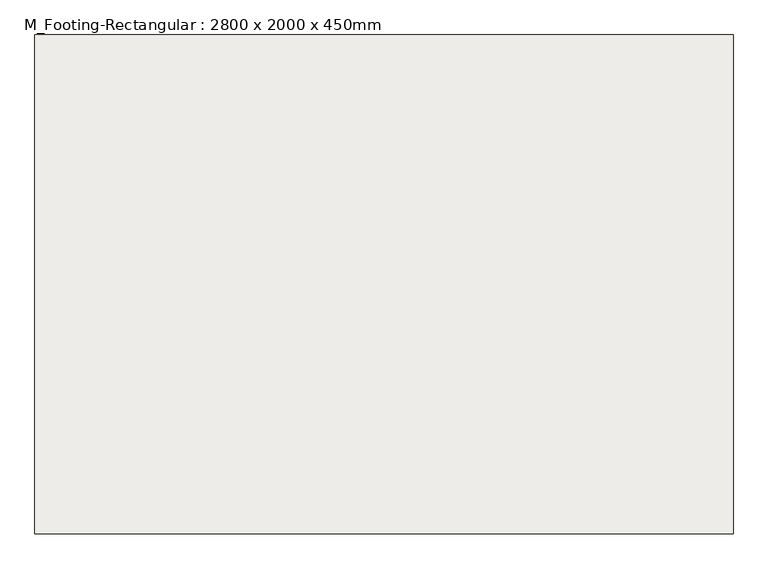
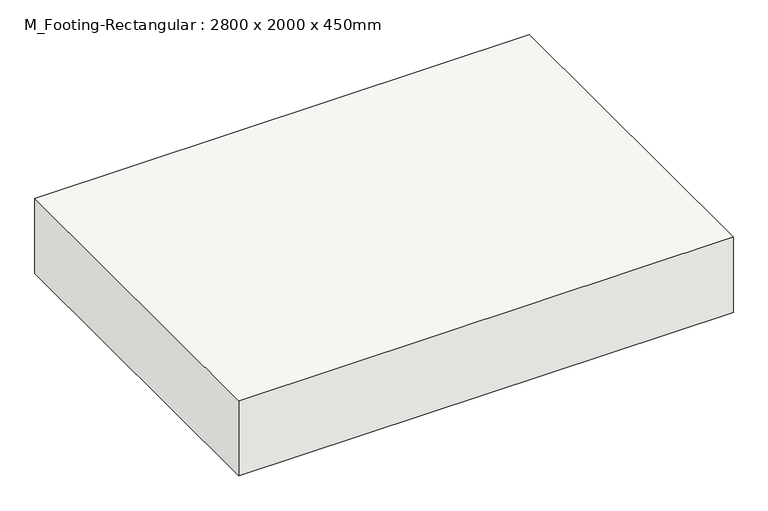
"""IFC4 building model written with IfcOpenShell, lengths in millimetres: slab geometry, M_Footing-Rectangular : 2800 x 2000 x 450mm."""

from ifc_helpers import new_model, si_unit, frame, origin, place, context, project, spatial, polyline, outline, extrude, source, transform, mapped, element, save


def m_footing_rectangular_2800_x_2000_x_450mm_3d0566a5(model_context):
    return source(origin(), model_context, "Body", "SweptSolid", [
        extrude(outline(polyline([(1400.0, 1000.0), (1400.0, -1000.0), (-1400.0, -1000.0), (-1400.0, 1000.0), (1400.0, 1000.0)])), frame((0.0, 0.0, -450.0), z_axis=(0.0, 0.0, 1.0), x_axis=(1.0, 0.0, 0.0)), (0.0, 0.0, 1.0), 450.0),
    ])


if __name__ == "__main__":
    model = new_model("IFC4")
    model_context = context("Model", 3, world=origin())
    ifc_project = project(units=[si_unit("LENGTHUNIT", "METRE", prefix="MILLI")], contexts=[model_context])
    site = spatial("IfcSite", under=ifc_project)
    building = spatial("IfcBuilding", under=site)
    placement = place(None, origin())
    m_footing_rectangular_2800_x_2000_x_450mm_shape = m_footing_rectangular_2800_x_2000_x_450mm_3d0566a5(model_context)
    element("IfcSlab", 1, ObjectType="M_Footing-Rectangular : 2800 x 2000 x 450mm", at=placement, inside=building, context=model_context, shape_type="MappedRepresentation", body=[
        mapped(m_footing_rectangular_2800_x_2000_x_450mm_shape, transform((0.0, 0.0, 0.0), x_axis=(1.0, 0.0, 0.0), y_axis=(0.0, 1.0, 0.0), z_axis=(0.0, 0.0, 1.0))),
    ])
    save(model, "model.ifc")

# Revit data of these elements
# Type "M_Footing-Rectangular : 2800 x 2000 x 450mm"
#   Width = 9' - 2.23622"
#   Length = 6' - 6.74016"
#   Foundation Thickness = 1' - 5.71654"
#   Structural Material [instance default] = Concrete, Cast-in-Place gray
#   Assembly Code = ""
# Element 1 (IfcSlab, "M_Footing-Rectangular : 2800 x 2000 x 450mm")
#   Materials on its faces: "Concrete, Cast-in-Place gray"
# Materials
#   "Concrete, Cast-in-Place gray": class "Concrete", colour RGB 192 192 192, transparency 0, Description = "Cast-in-place concrete", Cost = 0
